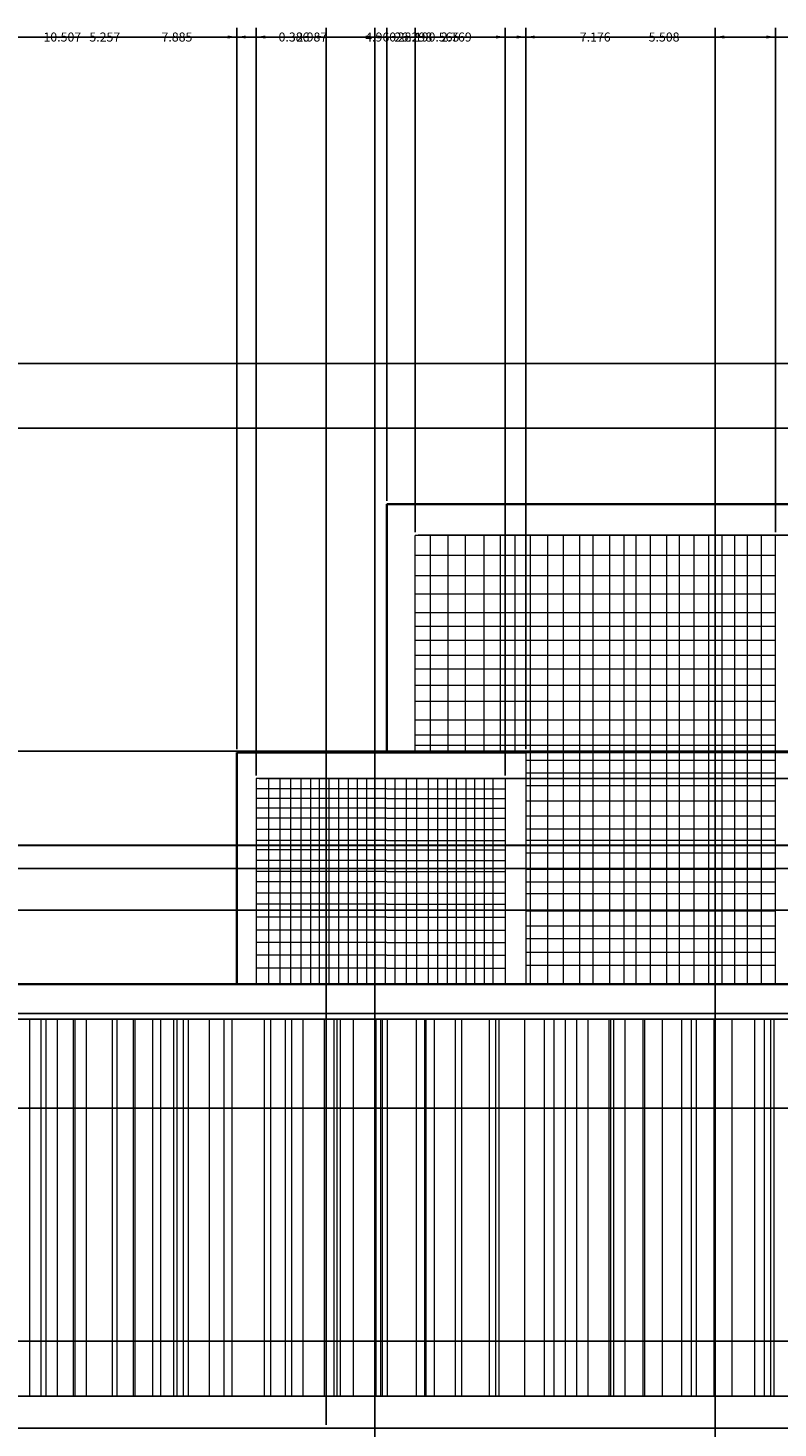
# Model space of a CAD drawing. Units: inches. Extents: x -10 to 130, y -32 to 34.
# Tile 18 of 22: x 75 to 90, y 6 to 34. Entities that reach past the tile are written whole.
import ezdxf

# ---------------------------------------------------------------- set-up
doc = ezdxf.new("R2010")
doc.units = ezdxf.units.IN
doc.header["$MEASUREMENT"] = 0
for name, color, linetype, lineweight in [('A-ANNO-DIMS', 2, 'Continuous', 18), ('A-ELEV', 7, 'Continuous', 35), ('A-GLAZ', 4, 'Continuous', 18)]:
    doc.layers.add(name, color=color, linetype=linetype, lineweight=lineweight)
doc.styles.get("Standard").update_dxf_attribs({"font": 'arial.ttf'})
doc.dimstyles.get("Standard").update_dxf_attribs({"dimtxt": 0.18, "dimasz": 0.18, "dimexe": 0.18, "dimexo": 0.0625, "dimgap": 0.09, "dimtad": 0, "dimtih": 1, "dimtoh": 1, "dimdec": 4, "dimzin": 0, "dimdsep": 46, "dimtxsty": 'Standard', "dimcen": 0.09, "dimadec": 0, "dimazin": 0, "dimtfac": 1, "dimtdec": 4, "dimtofl": 0, "dimtmove": 0, "dimatfit": 3, "dimfxl": 1, "dimtolj": 1, "dimtzin": 0, "dimarcsym": 0})

# ---------------------------------------------------------------- blocks, each defined once
blk = doc.blocks.new('*D2')
at = {"layer": 'A-ANNO-DIMS', "color": 0, "lineweight": -2, "transparency": 16777216}
for p, q in [((68.738, 27.199), (129.508, 27.199)), ((129.328, 27.019), (129.328, 3.074)), ((129.328, -21.234), (129.328, 2.71)), ((107.996, -21.414), (129.508, -21.414))]:
    blk.add_line(p, q, dxfattribs=at)
at = {"layer": 'A-ANNO-DIMS', "color": 0, "transparency": 16777216}
for points in [[(129.298, 27.019), (129.358, 27.019), (129.328, 27.199)], [(129.298, -21.234), (129.358, -21.234), (129.328, -21.414)]]:
    blk.add_solid(points, dxfattribs=at)
at = {"layer": 'Defpoints', "color": 0, "transparency": 16777216}
for p in [(68.676, 27.199), (129.328, 27.199), (107.933, -21.414)]:
    blk.add_point(p, dxfattribs=at)
at = {"layer": 'A-ANNO-DIMS', "color": 0, "transparency": 16777216, "insert": (129.328, 2.892), "char_height": 0.18, "attachment_point": 5}
blk.add_mtext('\\A1;48.61', dxfattribs=at)
blk = doc.blocks.new('*D9')
at = {"layer": 'A-ANNO-DIMS', "color": 0, "lineweight": -2, "transparency": 16777216}
for p, q in [((70.898, 6.07), (70.898, 33.879)), ((81.405, 6.07), (81.405, 33.879)), ((71.078, 33.699), (75.697, 33.699)), ((81.225, 33.699), (76.607, 33.699))]:
    blk.add_line(p, q, dxfattribs=at)
at = {"layer": 'A-ANNO-DIMS', "color": 0, "transparency": 16777216}
for points in [[(71.078, 33.729), (71.078, 33.669), (70.898, 33.699)], [(81.225, 33.729), (81.225, 33.669), (81.405, 33.699)]]:
    blk.add_solid(points, dxfattribs=at)
at = {"layer": 'Defpoints', "color": 0, "transparency": 16777216}
for p in [(81.405, 33.699), (70.898, 6.007), (81.405, 6.007)]:
    blk.add_point(p, dxfattribs=at)
at = {"layer": 'A-ANNO-DIMS', "color": 0, "transparency": 16777216, "insert": (76.152, 33.699), "char_height": 0.18, "attachment_point": 5}
blk.add_mtext('\\A1;10.507', dxfattribs=at)
blk = doc.blocks.new('*D21')
at = {"layer": 'A-ANNO-DIMS', "color": 0, "lineweight": -2, "transparency": 16777216}
for p, q in [((74.37, 17.67), (74.37, 33.879)), ((79.627, 19.52), (79.627, 33.879)), ((74.55, 33.699), (76.605, 33.699)), ((79.447, 33.699), (77.392, 33.699))]:
    blk.add_line(p, q, dxfattribs=at)
at = {"layer": 'A-ANNO-DIMS', "color": 0, "transparency": 16777216}
for points in [[(74.55, 33.729), (74.55, 33.669), (74.37, 33.699)], [(79.447, 33.729), (79.447, 33.669), (79.627, 33.699)]]:
    blk.add_solid(points, dxfattribs=at)
at = {"layer": 'Defpoints', "color": 0, "transparency": 16777216}
for p in [(79.627, 33.699), (79.627, 19.458), (74.37, 17.607)]:
    blk.add_point(p, dxfattribs=at)
at = {"layer": 'A-ANNO-DIMS', "color": 0, "transparency": 16777216, "insert": (76.998, 33.699), "char_height": 0.18, "attachment_point": 5}
blk.add_mtext('\\A1;5.257', dxfattribs=at)
blk = doc.blocks.new('*D22')
at = {"layer": 'A-ANNO-DIMS', "color": 0, "lineweight": -2, "transparency": 16777216}
for p, q in [((79.627, 19.52), (79.627, 33.879)), ((82.614, 24.464), (82.614, 33.879)), ((79.807, 33.699), (80.725, 33.699)), ((82.434, 33.699), (81.516, 33.699))]:
    blk.add_line(p, q, dxfattribs=at)
at = {"layer": 'A-ANNO-DIMS', "color": 0, "transparency": 16777216}
for points in [[(79.807, 33.729), (79.807, 33.669), (79.627, 33.699)], [(82.434, 33.729), (82.434, 33.669), (82.614, 33.699)]]:
    blk.add_solid(points, dxfattribs=at)
at = {"layer": 'Defpoints', "color": 0, "transparency": 16777216}
for p in [(82.614, 33.699), (82.614, 24.402), (79.627, 19.458)]:
    blk.add_point(p, dxfattribs=at)
at = {"layer": 'A-ANNO-DIMS', "color": 0, "transparency": 16777216, "insert": (81.121, 33.699), "char_height": 0.18, "attachment_point": 5}
blk.add_mtext('\\A1;2.987', dxfattribs=at)
blk = doc.blocks.new('*D23')
at = {"layer": 'A-ANNO-DIMS', "color": 0, "lineweight": -2, "transparency": 16777216}
for p, q in [((82.614, 24.464), (82.614, 33.879)), ((85.383, 19.52), (85.383, 33.879)), ((82.794, 33.699), (83.603, 33.699)), ((85.203, 33.699), (84.394, 33.699))]:
    blk.add_line(p, q, dxfattribs=at)
at = {"layer": 'A-ANNO-DIMS', "color": 0, "transparency": 16777216}
for points in [[(82.794, 33.729), (82.794, 33.669), (82.614, 33.699)], [(85.203, 33.729), (85.203, 33.669), (85.383, 33.699)]]:
    blk.add_solid(points, dxfattribs=at)
at = {"layer": 'Defpoints', "color": 0, "transparency": 16777216}
for p in [(85.383, 33.699), (82.614, 24.402), (85.383, 19.458)]:
    blk.add_point(p, dxfattribs=at)
at = {"layer": 'A-ANNO-DIMS', "color": 0, "transparency": 16777216, "insert": (83.999, 33.699), "char_height": 0.18, "attachment_point": 5}
blk.add_mtext('\\A1;2.769', dxfattribs=at)
blk = doc.blocks.new('*D24')
at = {"layer": 'A-ANNO-DIMS', "color": 0, "lineweight": -2, "transparency": 16777216}
for p, q in [((85.383, 19.52), (85.383, 33.879)), ((90.892, 24.464), (90.892, 33.879)), ((85.563, 33.699), (87.744, 33.699)), ((90.712, 33.699), (88.531, 33.699))]:
    blk.add_line(p, q, dxfattribs=at)
at = {"layer": 'A-ANNO-DIMS', "color": 0, "transparency": 16777216}
for points in [[(85.563, 33.729), (85.563, 33.669), (85.383, 33.699)], [(90.712, 33.729), (90.712, 33.669), (90.892, 33.699)]]:
    blk.add_solid(points, dxfattribs=at)
at = {"layer": 'Defpoints', "color": 0, "transparency": 16777216}
for p in [(90.892, 33.699), (90.892, 24.402), (85.383, 19.458)]:
    blk.add_point(p, dxfattribs=at)
at = {"layer": 'A-ANNO-DIMS', "color": 0, "transparency": 16777216, "insert": (88.138, 33.699), "char_height": 0.18, "attachment_point": 5}
blk.add_mtext('\\A1;5.508', dxfattribs=at)
blk = doc.blocks.new('*D29')
at = {"layer": 'A-ANNO-DIMS', "color": 0, "lineweight": -2, "transparency": 16777216}
for p, q in [((69.045, 14.903), (69.045, 33.879)), ((97.233, 14.903), (97.233, 33.879)), ((69.225, 33.699), (82.743, 33.699)), ((97.053, 33.699), (83.534, 33.699))]:
    blk.add_line(p, q, dxfattribs=at)
at = {"layer": 'A-ANNO-DIMS', "color": 0, "transparency": 16777216}
for points in [[(69.225, 33.729), (69.225, 33.669), (69.045, 33.699)], [(97.053, 33.729), (97.053, 33.669), (97.233, 33.699)]]:
    blk.add_solid(points, dxfattribs=at)
at = {"layer": 'Defpoints', "color": 0, "transparency": 16777216}
for p in [(97.233, 33.699), (69.045, 14.841), (97.233, 14.841)]:
    blk.add_point(p, dxfattribs=at)
at = {"layer": 'A-ANNO-DIMS', "color": 0, "transparency": 16777216, "insert": (83.139, 33.699), "char_height": 0.18, "attachment_point": 5}
blk.add_mtext('\\A1;28.19', dxfattribs=at)
blk = doc.blocks.new('*D60')
at = {"layer": 'A-ANNO-DIMS', "color": 0, "lineweight": -2, "transparency": 16777216}
for p, q in [((74.492, -13.293), (74.492, 33.879)), ((82.377, -15.202), (82.377, 33.879)), ((74.672, 33.699), (78.041, 33.699)), ((82.197, 33.699), (78.828, 33.699))]:
    blk.add_line(p, q, dxfattribs=at)
at = {"layer": 'A-ANNO-DIMS', "color": 0, "transparency": 16777216}
for points in [[(74.672, 33.729), (74.672, 33.669), (74.492, 33.699)], [(82.197, 33.729), (82.197, 33.669), (82.377, 33.699)]]:
    blk.add_solid(points, dxfattribs=at)
at = {"layer": 'Defpoints', "color": 0, "transparency": 16777216}
for p in [(82.377, 33.699), (74.492, -13.356), (82.377, -15.264)]:
    blk.add_point(p, dxfattribs=at)
at = {"layer": 'A-ANNO-DIMS', "color": 0, "transparency": 16777216, "insert": (78.435, 33.699), "char_height": 0.18, "attachment_point": 5}
blk.add_mtext('\\A1;7.885', dxfattribs=at)
blk = doc.blocks.new('*D66')
at = {"layer": 'A-ANNO-DIMS', "color": 0, "lineweight": -2, "transparency": 16777216}
for p, q in [((89.158, -16.844), (89.158, 33.879)), ((104.453, -13.219), (104.453, 33.879)), ((89.338, 33.699), (96.35, 33.699)), ((104.273, 33.699), (97.261, 33.699))]:
    blk.add_line(p, q, dxfattribs=at)
at = {"layer": 'A-ANNO-DIMS', "color": 0, "transparency": 16777216}
for points in [[(89.338, 33.729), (89.338, 33.669), (89.158, 33.699)], [(104.273, 33.729), (104.273, 33.669), (104.453, 33.699)]]:
    blk.add_solid(points, dxfattribs=at)
at = {"layer": 'Defpoints', "color": 0, "transparency": 16777216}
for p in [(104.453, 33.699), (104.453, -13.282), (89.158, -16.906)]:
    blk.add_point(p, dxfattribs=at)
at = {"layer": 'A-ANNO-DIMS', "color": 0, "transparency": 16777216, "insert": (96.805, 33.699), "char_height": 0.18, "attachment_point": 5}
blk.add_mtext('\\A1;15.295', dxfattribs=at)
blk = doc.blocks.new('*D79')
at = {"layer": 'A-ANNO-DIMS', "color": 0, "lineweight": -2, "transparency": 16777216}
for p, q in [((62.588, 7.736), (129.508, 7.736)), ((129.328, 7.556), (129.328, 5.559)), ((129.328, 3.198), (129.328, 5.195)), ((62.588, 3.018), (129.508, 3.018))]:
    blk.add_line(p, q, dxfattribs=at)
at = {"layer": 'A-ANNO-DIMS', "color": 0, "transparency": 16777216}
for points in [[(129.298, 7.556), (129.358, 7.556), (129.328, 7.736)], [(129.298, 3.198), (129.358, 3.198), (129.328, 3.018)]]:
    blk.add_solid(points, dxfattribs=at)
at = {"layer": 'Defpoints', "color": 0, "transparency": 16777216}
for p in [(62.526, 7.736), (129.328, 7.736), (62.526, 3.018)]:
    blk.add_point(p, dxfattribs=at)
at = {"layer": 'A-ANNO-DIMS', "color": 0, "transparency": 16777216, "insert": (129.328, 5.377), "char_height": 0.18, "attachment_point": 5}
blk.add_mtext('\\A1;4.718', dxfattribs=at)
blk = doc.blocks.new('*D80')
at = {"layer": 'A-ANNO-DIMS', "color": 0, "lineweight": -2, "transparency": 16777216}
for p, q in [((62.588, 12.373), (129.508, 12.373)), ((129.328, 12.193), (129.328, 10.237)), ((129.328, 7.916), (129.328, 9.873)), ((62.588, 7.736), (129.508, 7.736))]:
    blk.add_line(p, q, dxfattribs=at)
at = {"layer": 'A-ANNO-DIMS', "color": 0, "transparency": 16777216}
for points in [[(129.298, 12.193), (129.358, 12.193), (129.328, 12.373)], [(129.298, 7.916), (129.358, 7.916), (129.328, 7.736)]]:
    blk.add_solid(points, dxfattribs=at)
at = {"layer": 'Defpoints', "color": 0, "transparency": 16777216}
for p in [(62.526, 12.373), (129.328, 12.373), (62.526, 7.736)]:
    blk.add_point(p, dxfattribs=at)
at = {"layer": 'A-ANNO-DIMS', "color": 0, "transparency": 16777216, "insert": (129.328, 10.055), "char_height": 0.18, "attachment_point": 5}
blk.add_mtext('\\A1;4.64', dxfattribs=at)
blk = doc.blocks.new('*D81')
at = {"layer": 'A-ANNO-DIMS', "color": 0, "lineweight": -2, "transparency": 16777216}
for p, q in [((62.588, 16.317), (129.508, 16.317)), ((129.328, 16.137), (129.328, 14.527)), ((129.328, 12.553), (129.328, 14.163)), ((62.588, 12.373), (129.508, 12.373))]:
    blk.add_line(p, q, dxfattribs=at)
at = {"layer": 'A-ANNO-DIMS', "color": 0, "transparency": 16777216}
for points in [[(129.298, 16.137), (129.358, 16.137), (129.328, 16.317)], [(129.298, 12.553), (129.358, 12.553), (129.328, 12.373)]]:
    blk.add_solid(points, dxfattribs=at)
at = {"layer": 'Defpoints', "color": 0, "transparency": 16777216}
for p in [(62.526, 16.317), (129.328, 16.317), (62.526, 12.373)]:
    blk.add_point(p, dxfattribs=at)
at = {"layer": 'A-ANNO-DIMS', "color": 0, "transparency": 16777216, "insert": (129.328, 14.345), "char_height": 0.18, "attachment_point": 5}
blk.add_mtext('\\A1;3.94', dxfattribs=at)
blk = doc.blocks.new('*D82')
at = {"layer": 'A-ANNO-DIMS', "color": 0, "lineweight": -2, "transparency": 16777216}
for p, q in [((19.651, 19.485), (129.508, 19.485)), ((129.328, 19.305), (129.328, 18.728)), ((129.328, 17.787), (129.328, 18.364)), ((68.738, 17.607), (129.508, 17.607))]:
    blk.add_line(p, q, dxfattribs=at)
at = {"layer": 'A-ANNO-DIMS', "color": 0, "transparency": 16777216}
for points in [[(129.298, 19.305), (129.358, 19.305), (129.328, 19.485)], [(129.298, 17.787), (129.358, 17.787), (129.328, 17.607)]]:
    blk.add_solid(points, dxfattribs=at)
at = {"layer": 'Defpoints', "color": 0, "transparency": 16777216}
for p in [(19.588, 19.485), (68.676, 17.607), (129.328, 17.607)]:
    blk.add_point(p, dxfattribs=at)
at = {"layer": 'A-ANNO-DIMS', "color": 0, "transparency": 16777216, "insert": (129.328, 18.546), "char_height": 0.18, "attachment_point": 5}
blk.add_mtext('\\A1;1.877', dxfattribs=at)
blk = doc.blocks.new('*D85')
at = {"layer": 'A-ANNO-DIMS', "color": 0, "lineweight": -2, "transparency": 16777216}
for p, q in [((50.097, 27.199), (129.508, 27.199)), ((129.328, 27.019), (129.328, 26.738)), ((129.328, 26.093), (129.328, 26.374)), ((51.432, 25.913), (129.508, 25.913))]:
    blk.add_line(p, q, dxfattribs=at)
at = {"layer": 'A-ANNO-DIMS', "color": 0, "transparency": 16777216}
for points in [[(129.298, 27.019), (129.358, 27.019), (129.328, 27.199)], [(129.298, 26.093), (129.358, 26.093), (129.328, 25.913)]]:
    blk.add_solid(points, dxfattribs=at)
at = {"layer": 'Defpoints', "color": 0, "transparency": 16777216}
for p in [(50.035, 27.199), (129.328, 27.199), (51.37, 25.913)]:
    blk.add_point(p, dxfattribs=at)
at = {"layer": 'A-ANNO-DIMS', "color": 0, "transparency": 16777216, "insert": (129.328, 26.556), "char_height": 0.18, "attachment_point": 5}
blk.add_mtext('\\A1;1.286', dxfattribs=at)
blk = doc.blocks.new('*D108')
at = {"layer": 'A-ANNO-DIMS', "color": 0, "lineweight": -2, "transparency": 16777216}
for p, q in [((50.009, 14.841), (129.508, 14.841)), ((129.328, 14.841), (129.328, 15.021)), ((129.328, 15.021), (129.508, 15.021)), ((129.328, 14.436), (129.328, 14.661)), ((49.025, 14.256), (129.508, 14.256))]:
    blk.add_line(p, q, dxfattribs=at)
at = {"layer": 'A-ANNO-DIMS', "color": 0, "transparency": 16777216}
for points in [[(129.298, 14.661), (129.358, 14.661), (129.328, 14.841)], [(129.298, 14.436), (129.358, 14.436), (129.328, 14.256)]]:
    blk.add_solid(points, dxfattribs=at)
at = {"layer": 'Defpoints', "color": 0, "transparency": 16777216}
for p in [(49.946, 14.841), (129.328, 14.841), (48.963, 14.256)]:
    blk.add_point(p, dxfattribs=at)
at = {"layer": 'A-ANNO-DIMS', "color": 0, "transparency": 16777216, "insert": (129.902, 15.021), "char_height": 0.18, "attachment_point": 5}
blk.add_mtext('\\A1;0.585', dxfattribs=at)
blk = doc.blocks.new('*D137')
at = {"layer": 'A-ANNO-DIMS', "color": 0, "lineweight": -2, "transparency": 16777216}
for p, q in [((69.995, 14.206), (69.995, 33.879)), ((96.293, 14.206), (96.293, 33.879)), ((70.175, 33.699), (82.678, 33.699)), ((96.113, 33.699), (83.609, 33.699))]:
    blk.add_line(p, q, dxfattribs=at)
at = {"layer": 'A-ANNO-DIMS', "color": 0, "transparency": 16777216}
for points in [[(70.175, 33.729), (70.175, 33.669), (69.995, 33.699)], [(96.113, 33.729), (96.113, 33.669), (96.293, 33.699)]]:
    blk.add_solid(points, dxfattribs=at)
at = {"layer": 'Defpoints', "color": 0, "transparency": 16777216}
for p in [(96.293, 33.699), (69.995, 14.144), (96.293, 14.144)]:
    blk.add_point(p, dxfattribs=at)
at = {"layer": 'A-ANNO-DIMS', "color": 0, "transparency": 16777216, "insert": (83.144, 33.699), "char_height": 0.18, "attachment_point": 5}
blk.add_mtext('\\A1;26.298', dxfattribs=at)
blk = doc.blocks.new('*D138')
at = {"layer": 'A-ANNO-DIMS', "color": 0, "lineweight": -2, "transparency": 16777216}
for p, q in [((69.112, 14.841), (129.508, 14.841)), ((129.328, 14.841), (129.328, 15.021)), ((129.328, 15.021), (129.508, 15.021)), ((129.328, 14.324), (129.328, 14.661)), ((70.057, 14.144), (129.508, 14.144))]:
    blk.add_line(p, q, dxfattribs=at)
at = {"layer": 'A-ANNO-DIMS', "color": 0, "transparency": 16777216}
for points in [[(129.298, 14.661), (129.358, 14.661), (129.328, 14.841)], [(129.298, 14.324), (129.358, 14.324), (129.328, 14.144)]]:
    blk.add_solid(points, dxfattribs=at)
at = {"layer": 'Defpoints', "color": 0, "transparency": 16777216}
for p in [(69.05, 14.841), (129.328, 14.841), (69.995, 14.144)]:
    blk.add_point(p, dxfattribs=at)
at = {"layer": 'A-ANNO-DIMS', "color": 0, "transparency": 16777216, "insert": (129.901, 15.021), "char_height": 0.18, "attachment_point": 5}
blk.add_mtext('\\A1;0.697', dxfattribs=at)
blk = doc.blocks.new('*D139')
at = {"layer": 'A-ANNO-DIMS', "color": 0, "lineweight": -2, "transparency": 16777216}
for p, q in [((70.057, 6.643), (129.508, 6.643)), ((129.328, 6.463), (129.328, 6.187)), ((69.108, 6.007), (129.508, 6.007)), ((129.328, 6.007), (129.328, 5.827)), ((129.328, 5.827), (129.148, 5.827))]:
    blk.add_line(p, q, dxfattribs=at)
at = {"layer": 'A-ANNO-DIMS', "color": 0, "transparency": 16777216}
for points in [[(129.298, 6.463), (129.358, 6.463), (129.328, 6.643)], [(129.298, 6.187), (129.358, 6.187), (129.328, 6.007)]]:
    blk.add_solid(points, dxfattribs=at)
at = {"layer": 'Defpoints', "color": 0, "transparency": 16777216}
for p in [(69.995, 6.643), (69.045, 6.007), (129.328, 6.007)]:
    blk.add_point(p, dxfattribs=at)
at = {"layer": 'A-ANNO-DIMS', "color": 0, "transparency": 16777216, "insert": (128.754, 5.827), "char_height": 0.18, "attachment_point": 5}
blk.add_mtext('\\A1;0.636', dxfattribs=at)
blk = doc.blocks.new('*D143')
at = {"layer": 'A-ANNO-DIMS', "color": 0, "lineweight": -2, "transparency": 16777216}
for p, q in [((82.614, 24.464), (82.614, 33.879)), ((83.179, 23.841), (83.179, 33.879)), ((82.794, 33.699), (82.999, 33.699)), ((83.179, 33.699), (83.359, 33.699))]:
    blk.add_line(p, q, dxfattribs=at)
at = {"layer": 'A-ANNO-DIMS', "color": 0, "transparency": 16777216}
for points in [[(82.794, 33.729), (82.794, 33.669), (82.614, 33.699)], [(82.999, 33.729), (82.999, 33.669), (83.179, 33.699)]]:
    blk.add_solid(points, dxfattribs=at)
at = {"layer": 'Defpoints', "color": 0, "transparency": 16777216}
for p in [(83.179, 33.699), (82.614, 24.402), (83.179, 23.779)]:
    blk.add_point(p, dxfattribs=at)
at = {"layer": 'A-ANNO-DIMS', "color": 0, "transparency": 16777216, "insert": (83.753, 33.699), "char_height": 0.18, "attachment_point": 5}
blk.add_mtext('\\A1;0.565', dxfattribs=at)
blk = doc.blocks.new('*D144')
at = {"layer": 'A-ANNO-DIMS', "color": 0, "lineweight": -2, "transparency": 16777216}
for p, q in [((83.179, 23.841), (83.179, 33.879)), ((90.355, 23.841), (90.355, 33.879)), ((83.359, 33.699), (86.374, 33.699)), ((90.175, 33.699), (87.16, 33.699))]:
    blk.add_line(p, q, dxfattribs=at)
at = {"layer": 'A-ANNO-DIMS', "color": 0, "transparency": 16777216}
for points in [[(83.359, 33.729), (83.359, 33.669), (83.179, 33.699)], [(90.175, 33.729), (90.175, 33.669), (90.355, 33.699)]]:
    blk.add_solid(points, dxfattribs=at)
at = {"layer": 'Defpoints', "color": 0, "transparency": 16777216}
for p in [(90.355, 33.699), (83.179, 23.779), (90.355, 23.779)]:
    blk.add_point(p, dxfattribs=at)
at = {"layer": 'A-ANNO-DIMS', "color": 0, "transparency": 16777216, "insert": (86.767, 33.699), "char_height": 0.18, "attachment_point": 5}
blk.add_mtext('\\A1;7.176', dxfattribs=at)
blk = doc.blocks.new('*D145')
at = {"layer": 'A-ANNO-DIMS', "color": 0, "lineweight": -2, "transparency": 16777216}
for p, q in [((129.328, 24.402), (129.328, 24.582)), ((129.328, 24.582), (129.508, 24.582)), ((82.677, 24.402), (129.508, 24.402)), ((129.328, 23.959), (129.328, 24.222)), ((83.241, 23.779), (129.508, 23.779))]:
    blk.add_line(p, q, dxfattribs=at)
at = {"layer": 'A-ANNO-DIMS', "color": 0, "transparency": 16777216}
for points in [[(129.298, 24.222), (129.358, 24.222), (129.328, 24.402)], [(129.298, 23.959), (129.358, 23.959), (129.328, 23.779)]]:
    blk.add_solid(points, dxfattribs=at)
at = {"layer": 'Defpoints', "color": 0, "transparency": 16777216}
for p in [(82.614, 24.402), (129.328, 24.402), (83.179, 23.779)]:
    blk.add_point(p, dxfattribs=at)
at = {"layer": 'A-ANNO-DIMS', "color": 0, "transparency": 16777216, "insert": (129.901, 24.582), "char_height": 0.18, "attachment_point": 5}
blk.add_mtext('\\A1;0.623', dxfattribs=at)
blk = doc.blocks.new('*D146')
at = {"layer": 'A-ANNO-DIMS', "color": 0, "lineweight": -2, "transparency": 16777216}
for p, q in [((79.627, 19.52), (79.627, 33.879)), ((80.013, 18.998), (80.013, 33.879)), ((79.447, 33.699), (79.267, 33.699)), ((80.193, 33.699), (80.373, 33.699))]:
    blk.add_line(p, q, dxfattribs=at)
at = {"layer": 'A-ANNO-DIMS', "color": 0, "transparency": 16777216}
for points in [[(79.447, 33.729), (79.447, 33.669), (79.627, 33.699)], [(80.193, 33.729), (80.193, 33.669), (80.013, 33.699)]]:
    blk.add_solid(points, dxfattribs=at)
at = {"layer": 'Defpoints', "color": 0, "transparency": 16777216}
for p in [(80.013, 33.699), (79.627, 19.458), (80.013, 18.936)]:
    blk.add_point(p, dxfattribs=at)
at = {"layer": 'A-ANNO-DIMS', "color": 0, "transparency": 16777216, "insert": (80.766, 33.699), "char_height": 0.18, "attachment_point": 5}
blk.add_mtext('\\A1;0.386', dxfattribs=at)
blk = doc.blocks.new('*D147')
at = {"layer": 'A-ANNO-DIMS', "color": 0, "lineweight": -2, "transparency": 16777216}
for p, q in [((80.013, 18.998), (80.013, 33.879)), ((84.973, 18.998), (84.973, 33.879)), ((80.193, 33.699), (82.096, 33.699)), ((84.793, 33.699), (82.89, 33.699))]:
    blk.add_line(p, q, dxfattribs=at)
at = {"layer": 'A-ANNO-DIMS', "color": 0, "transparency": 16777216}
for points in [[(80.193, 33.729), (80.193, 33.669), (80.013, 33.699)], [(84.793, 33.729), (84.793, 33.669), (84.973, 33.699)]]:
    blk.add_solid(points, dxfattribs=at)
at = {"layer": 'Defpoints', "color": 0, "transparency": 16777216}
for p in [(84.973, 33.699), (80.013, 18.936), (84.973, 18.936)]:
    blk.add_point(p, dxfattribs=at)
at = {"layer": 'A-ANNO-DIMS', "color": 0, "transparency": 16777216, "insert": (82.493, 33.699), "char_height": 0.18, "attachment_point": 5}
blk.add_mtext('\\A1;4.960', dxfattribs=at)
blk = doc.blocks.new('*D148')
at = {"layer": 'A-ANNO-DIMS', "color": 0, "lineweight": -2, "transparency": 16777216}
for p, q in [((129.327673, 19.637521), (129.327673, 19.817521)), ((79.689531, 19.457521), (129.507673, 19.457521)), ((80.07533, 18.935883), (129.507673, 18.935883)), ((129.327673, 18.755883), (129.327673, 18.575883))]:
    blk.add_line(p, q, dxfattribs=at)
at = {"layer": 'A-ANNO-DIMS', "color": 0, "transparency": 16777216}
for points in [[(129.297673, 19.637521), (129.357673, 19.637521), (129.327673, 19.457521)], [(129.297673, 18.755883), (129.357673, 18.755883), (129.327673, 18.935883)]]:
    blk.add_solid(points, dxfattribs=at)
at = {"layer": 'Defpoints', "color": 0, "transparency": 16777216}
for p in [(79.627031, 19.457521), (129.327673, 19.457521), (80.01283, 18.935883)]:
    blk.add_point(p, dxfattribs=at)
at = {"layer": 'A-ANNO-DIMS', "color": 0, "transparency": 16777216, "insert": (129.327673, 19.196702), "char_height": 0.18, "attachment_point": 5}
blk.add_mtext('\\A1;0.522', dxfattribs=at)
blk = doc.blocks.new('*D150')
at = {"layer": 'A-ANNO-DIMS', "color": 0, "lineweight": -2, "transparency": 16777216}
for p, q in [((129.327673, 17.787359), (129.327673, 17.967359)), ((74.432221, 17.607359), (129.507673, 17.607359)), ((73.944831, 17.142679), (129.507673, 17.142679)), ((129.327673, 16.962679), (129.327673, 16.782679))]:
    blk.add_line(p, q, dxfattribs=at)
at = {"layer": 'A-ANNO-DIMS', "color": 0, "transparency": 16777216}
for points in [[(129.297673, 17.787359), (129.357673, 17.787359), (129.327673, 17.607359)], [(129.297673, 16.962679), (129.357673, 16.962679), (129.327673, 17.142679)]]:
    blk.add_solid(points, dxfattribs=at)
at = {"layer": 'Defpoints', "color": 0, "transparency": 16777216}
for p in [(74.369721, 17.607359), (129.327673, 17.607359), (73.882331, 17.142679)]:
    blk.add_point(p, dxfattribs=at)
at = {"layer": 'A-ANNO-DIMS', "color": 0, "transparency": 16777216, "insert": (129.327673, 17.375019), "char_height": 0.18, "attachment_point": 5}
blk.add_mtext('\\A1;0.465', dxfattribs=at)
blk = doc.blocks.new('*D154')
at = {"layer": 'A-ANNO-DIMS', "color": 0, "lineweight": -2, "transparency": 16777216}
for p, q in [((81.468, 6.007), (129.508, 6.007)), ((129.328, 5.827), (129.328, 3.941)), ((129.328, 1.691), (129.328, 3.577)), ((81.468, 1.511), (129.508, 1.511))]:
    blk.add_line(p, q, dxfattribs=at)
at = {"layer": 'A-ANNO-DIMS', "color": 0, "transparency": 16777216}
for points in [[(129.298, 5.827), (129.358, 5.827), (129.328, 6.007)], [(129.298, 1.691), (129.358, 1.691), (129.328, 1.511)]]:
    blk.add_solid(points, dxfattribs=at)
at = {"layer": 'Defpoints', "color": 0, "transparency": 16777216}
for p in [(81.405, 6.007), (129.328, 6.007), (81.405, 1.511)]:
    blk.add_point(p, dxfattribs=at)
at = {"layer": 'A-ANNO-DIMS', "color": 0, "transparency": 16777216, "insert": (129.328, 3.759), "char_height": 0.18, "attachment_point": 5}
blk.add_mtext('\\A1;4.497', dxfattribs=at)

msp = doc.modelspace()

# ---------------------------------------------------------------- linework, layer by layer
at = {"layer": 'A-ELEV'}
for p, q in [((90.8917, 24.4019), (82.6141, 24.4019)), ((82.6141, 24.4019), (82.6141, 19.4575)), ((82.6141, 19.4575), (79.627, 19.4575)), ((79.627, 19.4575), (79.627, 14.8409)), ((82.6141, 19.4575), (85.3833, 19.4575)), ((97.276, 14.8409), (69.0452, 14.8409))]:
    msp.add_line(p, q, dxfattribs=at)
at = {"layer": 'A-GLAZ'}
for p, q in [((83.1789, 19.4575), (83.1789, 23.7785)), ((90.3554, 23.7785), (83.1789, 23.7785)), ((83.4866, 19.4575), (83.4866, 23.7785)), ((83.8354, 19.4575), (83.8354, 23.7785)), ((84.1841, 19.4575), (84.1841, 23.7785)), ((84.5534, 19.4575), (84.5534, 23.7785)), ((84.8816, 19.4575), (84.8816, 23.7785)), ((85.1688, 19.4575), (85.1688, 23.7785)), ((85.4766, 14.8409), (85.4766, 23.7785)), ((85.8253, 14.8409), (85.8253, 23.7785)), ((86.133, 14.8409), (86.133, 23.7785)), ((86.4613, 14.8409), (86.4613, 23.7785)), ((86.7279, 14.8409), (86.7279, 23.7785)), ((87.0562, 14.8409), (87.0562, 23.7785)), ((87.3434, 14.8409), (87.3434, 23.7785)), ((87.5816, 14.8409), (87.5816, 23.7785)), ((87.8659, 14.8409), (87.8659, 23.7785)), ((88.1922, 14.8409), (88.1922, 23.7785)), ((88.4452, 14.8409), (88.4452, 23.7785)), ((88.7362, 14.8409), (88.7362, 23.7785)), ((89.0271, 14.8409), (89.0271, 23.7785)), ((89.2928, 14.8409), (89.2928, 23.7785)), ((89.5458, 14.8409), (89.5458, 23.7785)), ((89.7988, 14.8409), (89.7988, 23.7785)), ((90.0771, 14.8409), (90.0771, 23.7785)), ((90.3554, 14.8409), (90.3554, 23.7785)), ((90.3554, 23.3752), (83.1789, 23.3752)), ((90.3554, 22.9718), (83.1789, 22.9718)), ((90.3554, 22.6051), (83.1789, 22.6051)), ((90.3554, 22.2381), (83.1789, 22.2381)), ((90.3554, 21.9622), (83.1789, 21.9622)), ((90.3554, 21.6862), (83.1789, 21.6862)), ((90.3554, 21.3872), (83.1789, 21.3872)), ((90.3554, 21.1112), (83.1789, 21.1112)), ((90.3554, 20.7893), (83.1789, 20.7893)), ((90.3554, 20.4673), (83.1789, 20.4673)), ((90.3554, 20.0993), (83.1789, 20.0993)), ((90.3554, 19.8003), (83.1789, 19.8003)), ((90.3554, 19.5933), (83.1789, 19.5933)), ((85.3833, 19.4575), (85.3833, 14.8409)), ((90.3554, 19.2944), (85.3833, 19.2944)), ((90.3554, 19.0414), (85.3833, 19.0414)), ((82.6141, 18.9359), (80.0128, 18.9359)), ((80.0128, 18.9359), (80.0128, 14.8409)), ((82.6141, 18.7336), (80.0128, 18.7336)), ((80.2574, 18.9359), (80.2574, 14.8409)), ((80.4844, 18.9359), (80.4844, 14.8409)), ((80.694, 18.9359), (80.694, 14.8409)), ((80.9036, 18.9359), (80.9036, 14.8409)), ((81.0958, 18.9359), (81.0958, 14.8409)), ((81.2704, 18.9359), (81.2704, 14.8409)), ((81.4626, 18.9359), (81.4626, 14.8409)), ((81.6547, 18.9359), (81.6547, 14.8409)), ((81.8468, 18.9359), (81.8468, 14.8409)), ((82.0215, 18.9359), (82.0215, 14.8409)), ((82.2136, 18.9359), (82.2136, 14.8409)), ((82.3708, 18.9359), (82.3708, 14.8409)), ((82.5804, 18.9359), (82.5804, 14.8409)), ((82.6141, 18.9359), (84.9733, 18.9359)), ((82.6141, 18.7336), (84.9733, 18.7336)), ((82.7725, 18.9359), (82.7725, 14.8409)), ((82.9996, 18.9359), (82.9996, 14.8409)), ((83.2092, 18.9359), (83.2092, 14.8409)), ((83.436, 18.9359), (83.436, 14.8409)), ((83.6281, 18.9359), (83.6281, 14.8409)), ((83.8202, 18.9359), (83.8202, 14.8409)), ((83.9949, 18.9359), (83.9949, 14.8409)), ((84.187, 18.9359), (84.187, 14.8409)), ((84.3617, 18.9359), (84.3617, 14.8409)), ((84.5538, 18.9359), (84.5538, 14.8409)), ((84.7285, 18.9359), (84.7285, 14.8409)), ((84.9733, 18.9359), (84.9733, 14.8409)), ((90.3554, 18.7884), (85.3833, 18.7884)), ((82.6141, 18.5419), (80.0128, 18.5419)), ((82.6141, 18.5419), (84.9733, 18.5419)), ((90.3554, 18.4894), (85.3833, 18.4894)), ((82.6141, 18.3502), (80.0128, 18.3502)), ((82.6141, 18.1479), (80.0128, 18.1479)), ((82.6141, 18.3502), (84.9733, 18.3502)), ((82.6141, 18.1479), (84.9733, 18.1479)), ((90.3554, 18.1847), (85.3833, 18.1847)), ((82.6141, 17.9243), (80.0128, 17.9243)), ((82.6141, 17.9243), (84.9733, 17.9243)), ((90.3554, 17.9317), (85.3833, 17.9317)), ((82.6141, 17.7007), (80.0128, 17.7007)), ((82.6141, 17.7007), (84.9733, 17.7007)), ((90.3554, 17.7017), (85.3833, 17.7017)), ((82.6141, 17.5197), (80.0128, 17.5197)), ((82.6141, 17.3067), (80.0128, 17.3067)), ((82.6141, 17.5197), (84.9733, 17.5197)), ((82.6141, 17.3067), (84.9733, 17.3067)), ((90.3554, 17.4487), (85.3833, 17.4487)), ((82.6141, 17.0831), (80.0128, 17.0831)), ((82.6141, 17.0831), (84.9733, 17.0831)), ((90.3554, 17.1267), (85.3833, 17.1267)), ((82.6141, 16.8808), (80.0128, 16.8808)), ((82.6141, 16.8808), (84.9733, 16.8808)), ((90.3554, 16.8738), (85.3833, 16.8738)), ((82.6141, 16.6571), (80.0128, 16.6571)), ((82.6141, 16.6571), (84.9733, 16.6571)), ((90.3554, 16.6438), (85.3833, 16.6438)), ((82.6141, 16.4335), (80.0128, 16.4335)), ((82.6141, 16.1747), (80.0128, 16.1747)), ((82.6141, 16.4335), (84.9733, 16.4335)), ((82.6141, 16.1747), (84.9733, 16.1747)), ((90.3554, 16.2988), (85.3833, 16.2988)), ((82.6141, 15.9192), (80.0128, 15.9192)), ((82.6141, 15.9192), (84.9733, 15.9192)), ((90.3554, 15.9998), (85.3833, 15.9998)), ((82.6141, 15.6742), (80.0128, 15.6742)), ((82.6141, 15.6742), (84.9733, 15.6742)), ((90.3554, 15.7469), (85.3833, 15.7469)), ((82.6141, 15.4187), (80.0128, 15.4187)), ((82.6141, 15.4187), (84.9733, 15.4187)), ((90.3554, 15.4709), (85.3833, 15.4709)), ((82.6141, 15.1631), (80.0128, 15.1631)), ((82.6141, 15.1631), (84.9733, 15.1631)), ((90.3554, 15.2179), (85.3833, 15.2179)), ((96.2927, 14.144), (69.9946, 14.144)), ((75.5056, 6.6433), (75.5056, 14.144)), ((75.7312, 6.6433), (75.7312, 14.144)), ((75.8279, 6.6433), (75.8279, 14.144)), ((76.0535, 6.6433), (76.0535, 14.144)), ((76.0535, 6.6433), (76.0535, 14.144)), ((76.3758, 6.6433), (76.3758, 14.144)), ((76.408, 6.6433), (76.408, 14.144)), ((76.6336, 6.6433), (76.6336, 14.144)), ((77.1492, 6.6433), (77.1492, 14.144)), ((77.2459, 6.6433), (77.2459, 14.144)), ((77.5682, 6.6433), (77.5682, 14.144)), ((77.6004, 6.6433), (77.6004, 14.144)), ((77.955, 6.6433), (77.955, 14.144)), ((78.1161, 6.6433), (78.1161, 14.144)), ((78.1161, 6.6433), (78.1161, 14.144)), ((78.3739, 6.6433), (78.3739, 14.144)), ((78.4384, 6.6433), (78.4384, 14.144)), ((78.5673, 6.6433), (78.5673, 14.144)), ((78.664, 6.6433), (78.664, 14.144)), ((79.0829, 6.6433), (79.0829, 14.144)), ((79.373, 6.6433), (79.373, 14.144)), ((79.5341, 6.6433), (79.5341, 14.144)), ((80.1787, 6.6433), (80.1787, 14.144)), ((80.3076, 6.6433), (80.3076, 14.144)), ((80.5977, 6.6433), (80.5977, 14.144)), ((80.5977, 6.6433), (80.5977, 14.144)), ((80.7266, 6.6433), (80.7266, 14.144)), ((80.9522, 6.6433), (80.9522, 14.144)), ((81.3711, 6.6433), (81.3711, 14.144)), ((81.5645, 6.6433), (81.5645, 14.144)), ((81.629, 6.6433), (81.629, 14.144)), ((81.6934, 6.6433), (81.6934, 14.144)), ((81.9512, 6.6433), (81.9512, 14.144)), ((82.4024, 6.6433), (82.4024, 14.144)), ((82.4991, 6.6433), (82.4991, 14.144)), ((82.5313, 6.6433), (82.5313, 14.144)), ((82.628, 6.6433), (82.628, 14.144)), ((83.2081, 6.6433), (83.2081, 14.144)), ((83.3693, 6.6433), (83.3693, 14.144)), ((83.4015, 6.6433), (83.4015, 14.144)), ((83.5626, 6.6433), (83.5626, 14.144)), ((83.9816, 6.6433), (83.9816, 14.144)), ((83.9816, 6.6433), (83.9816, 14.144)), ((84.1105, 6.6433), (84.1105, 14.144)), ((84.6584, 6.6433), (84.6584, 14.144)), ((84.6584, 6.6433), (84.6584, 14.144)), ((84.7873, 6.6433), (84.7873, 14.144)), ((84.8518, 6.6433), (84.8518, 14.144)), ((85.3674, 6.6433), (85.3674, 14.144)), ((85.7542, 6.6433), (85.7542, 14.144)), ((85.7542, 6.6433), (85.7542, 14.144)), ((85.9475, 6.6433), (85.9475, 14.144)), ((86.1731, 6.6433), (86.1731, 14.144)), ((86.3987, 6.6433), (86.3987, 14.144)), ((86.6243, 6.6433), (86.6243, 14.144)), ((87.0433, 6.6433), (87.0433, 14.144)), ((87.0755, 6.6433), (87.0755, 14.144)), ((87.14, 6.6433), (87.14, 14.144)), ((87.3656, 6.6433), (87.3656, 14.144)), ((87.7201, 6.6433), (87.7201, 14.144)), ((87.7523, 6.6433), (87.7523, 14.144)), ((88.1068, 6.6433), (88.1068, 14.144)), ((88.4935, 6.6433), (88.4935, 14.144)), ((88.6869, 6.6433), (88.6869, 14.144)), ((88.7836, 6.6433), (88.7836, 14.144)), ((89.1381, 6.6433), (89.1381, 14.144)), ((89.4926, 6.6433), (89.4926, 14.144)), ((89.9438, 6.6433), (89.9438, 14.144)), ((90.1372, 6.6433), (90.1372, 14.144)), ((90.2661, 6.6433), (90.2661, 14.144)), ((90.3305, 6.6433), (90.3305, 14.144)), ((96.2927, 6.6433), (69.9946, 6.6433))]:
    msp.add_line(p, q, dxfattribs=at)

# ---------------------------------------------------------------- dimensions: what is measured, and where the dimension line sits
at = {"layer": 'A-ANNO-DIMS'}
for base, p1, p2, override, picture, middle in [((97.2325, 33.6987), (69.0452, 14.8409), (97.2325, 14.8409), {"dimdec": 2, "dimlfac": 1, "dimrnd": 0, "dimzin": 0, "dimdsep": 46, "dimlunit": 2}, '*D29', (83.1389, 33.6987)), ((96.2927, 33.6987), (69.9946, 14.144), (96.2927, 14.144), {"dimdec": 3, "dimlfac": 1, "dimrnd": 0, "dimzin": 0, "dimdsep": 46, "dimlunit": 2}, '*D137', (83.1437, 33.6987)), ((81.4053, 33.6987), (70.898, 6.0074), (81.4053, 6.0074), {"dimdec": 3, "dimlfac": 1, "dimrnd": 0, "dimzin": 0, "dimdsep": 46, "dimlunit": 2}, '*D9', (76.1517, 33.6987)), ((79.627, 33.6987), (74.3697, 17.6074), (79.627, 19.4575), {"dimdec": 3, "dimlfac": 1, "dimrnd": 0, "dimzin": 0, "dimdsep": 46, "dimlunit": 2}, '*D21', (76.9984, 33.6987)), ((82.377, 33.6987), (74.492, -13.3558), (82.377, -15.2645), {"dimdec": 3, "dimlfac": 1, "dimrnd": 0, "dimzin": 0, "dimdsep": 46, "dimlunit": 2}, '*D60', (78.4345, 33.6987)), ((80.0128, 33.6987), (79.627, 19.4575), (80.0128, 18.9359), {"dimdec": 3, "dimlfac": 1, "dimrnd": 0, "dimzin": 0, "dimdsep": 46, "dimlunit": 2}, '*D146', (80.7665, 33.6987)), ((82.6141, 33.6987), (79.627, 19.4575), (82.6141, 24.4019), {"dimdec": 3, "dimlfac": 1, "dimrnd": 0, "dimzin": 0, "dimdsep": 46, "dimlunit": 2}, '*D22', (81.1206, 33.6987)), ((84.97332, 33.69866), (80.01283, 18.93588), (84.97332, 18.93588), {"dimdec": 3, "dimlfac": 1, "dimrnd": 0, "dimzin": 0, "dimdsep": 46, "dimlunit": 2}, '*D147', (82.49308, 33.69866)), ((85.3833, 33.6987), (82.6141, 24.4019), (85.3833, 19.4575), {"dimdec": 3, "dimlfac": 1, "dimrnd": 0, "dimzin": 0, "dimdsep": 46, "dimlunit": 2}, '*D23', (83.9987, 33.6987)), ((83.1789, 33.6987), (82.6141, 24.4019), (83.1789, 23.7785), {"dimdec": 3, "dimlfac": 1, "dimrnd": 0, "dimzin": 0, "dimdsep": 46, "dimlunit": 2}, '*D143', (83.7533, 33.6987)), ((90.35537, 33.69866), (83.17891, 23.77854), (90.35537, 23.77854), {"dimdec": 3, "dimlfac": 1, "dimrnd": 0, "dimzin": 0, "dimdsep": 46, "dimlunit": 2}, '*D144', (86.76714, 33.69866)), ((90.8917, 33.6987), (85.3833, 19.4575), (90.8917, 24.4019), {"dimdec": 3, "dimlfac": 1, "dimrnd": 0, "dimzin": 0, "dimdsep": 46, "dimlunit": 2}, '*D24', (88.1375, 33.6987)), ((104.4531, 33.6987), (89.1578, -16.9063), (104.4531, -13.2819), {"dimdec": 3, "dimlfac": 1, "dimrnd": 0, "dimzin": 0, "dimdsep": 46, "dimlunit": 2}, '*D66', (96.8055, 33.6987))]:
    dim = msp.add_linear_dim(base=base, p1=p1, p2=p2, dimstyle='Standard', override=override, dxfattribs=at)
    dim.commit()
    dim.dimension.update_dxf_attribs({"geometry": picture, "text_midpoint": middle})
for base, p1, p2, override, picture, middle in [((129.3277, 27.1987), (51.3699, 25.9127), (50.0347, 27.1987), {"dimdec": 3, "dimlfac": 1, "dimrnd": 0, "dimzin": 0, "dimdsep": 46, "dimlunit": 2}, '*D85', (129.3277, 26.5557)), ((129.3277, 27.1987), (107.9333, -21.4145), (68.6759, 27.1987), {"dimdec": 2, "dimlfac": 1, "dimrnd": 0, "dimzin": 0, "dimdsep": 46, "dimlunit": 2}, '*D2', (129.3277, 2.8921)), ((129.3277, 24.4019), (83.1789, 23.7785), (82.6141, 24.4019), {"dimdec": 3, "dimlfac": 1, "dimrnd": 0, "dimzin": 0, "dimdsep": 46, "dimlunit": 2}, '*D145', (129.9014, 24.5819)), ((129.3277, 19.4575), (80.0128, 18.9359), (79.627, 19.4575), {"dimdec": 3, "dimlfac": 1, "dimrnd": 0, "dimzin": 0, "dimdsep": 46, "dimlunit": 2}, '*D148', (129.3277, 19.1967)), ((129.3277, 17.6074), (19.5881, 19.4845), (68.6759, 17.6074), {"dimdec": 3, "dimlfac": 1, "dimrnd": 0, "dimzin": 0, "dimdsep": 46, "dimlunit": 2}, '*D82', (129.3277, 18.5459)), ((129.3277, 17.6074), (73.8823, 17.1427), (74.3697, 17.6074), {"dimdec": 3, "dimlfac": 1, "dimrnd": 0, "dimzin": 0, "dimdsep": 46, "dimlunit": 2}, '*D150', (129.3277, 17.375)), ((129.3277, 16.3174), (62.5256, 12.3729), (62.5256, 16.3174), {"dimdec": 2, "dimlfac": 1, "dimrnd": 0, "dimzin": 0, "dimdsep": 46, "dimlunit": 2}, '*D81', (129.3277, 14.3452)), ((129.3277, 14.8409), (48.963, 14.2556), (49.9462, 14.8409), {"dimdec": 3, "dimlfac": 1, "dimrnd": 0, "dimzin": 0, "dimdsep": 46, "dimlunit": 2}, '*D108', (129.9021, 15.0209)), ((129.3277, 14.8409), (69.9946, 14.144), (69.0498, 14.8409), {"dimdec": 3, "dimlfac": 1, "dimrnd": 0, "dimzin": 0, "dimdsep": 46, "dimlunit": 2}, '*D138', (129.9014, 15.0209)), ((129.3277, 12.3729), (62.5256, 7.7364), (62.5256, 12.3729), {"dimdec": 2, "dimlfac": 1, "dimrnd": 0, "dimzin": 0, "dimdsep": 46, "dimlunit": 2}, '*D80', (129.3277, 10.0547)), ((129.3277, 7.7364), (62.5256, 3.0181), (62.5256, 7.7364), {"dimdec": 3, "dimlfac": 1, "dimrnd": 0, "dimzin": 0, "dimdsep": 46, "dimlunit": 2}, '*D79', (129.3277, 5.3773)), ((129.3277, 6.0074), (69.9946, 6.6433), (69.0452, 6.0074), {"dimdec": 3, "dimlfac": 1, "dimrnd": 0, "dimzin": 0, "dimdsep": 46, "dimlunit": 2}, '*D139', (128.754, 5.8274)), ((129.3277, 6.0074), (81.4053, 1.5107), (81.4053, 6.0074), {"dimdec": 3, "dimlfac": 1, "dimrnd": 0, "dimzin": 0, "dimdsep": 46, "dimlunit": 2}, '*D154', (129.3277, 3.7591))]:
    dim = msp.add_linear_dim(base=base, p1=p1, p2=p2, angle=90, dimstyle='Standard', override=override, dxfattribs=at)
    dim.commit()
    dim.dimension.update_dxf_attribs({"geometry": picture, "text_midpoint": middle})

doc.saveas('drawing.dxf')
